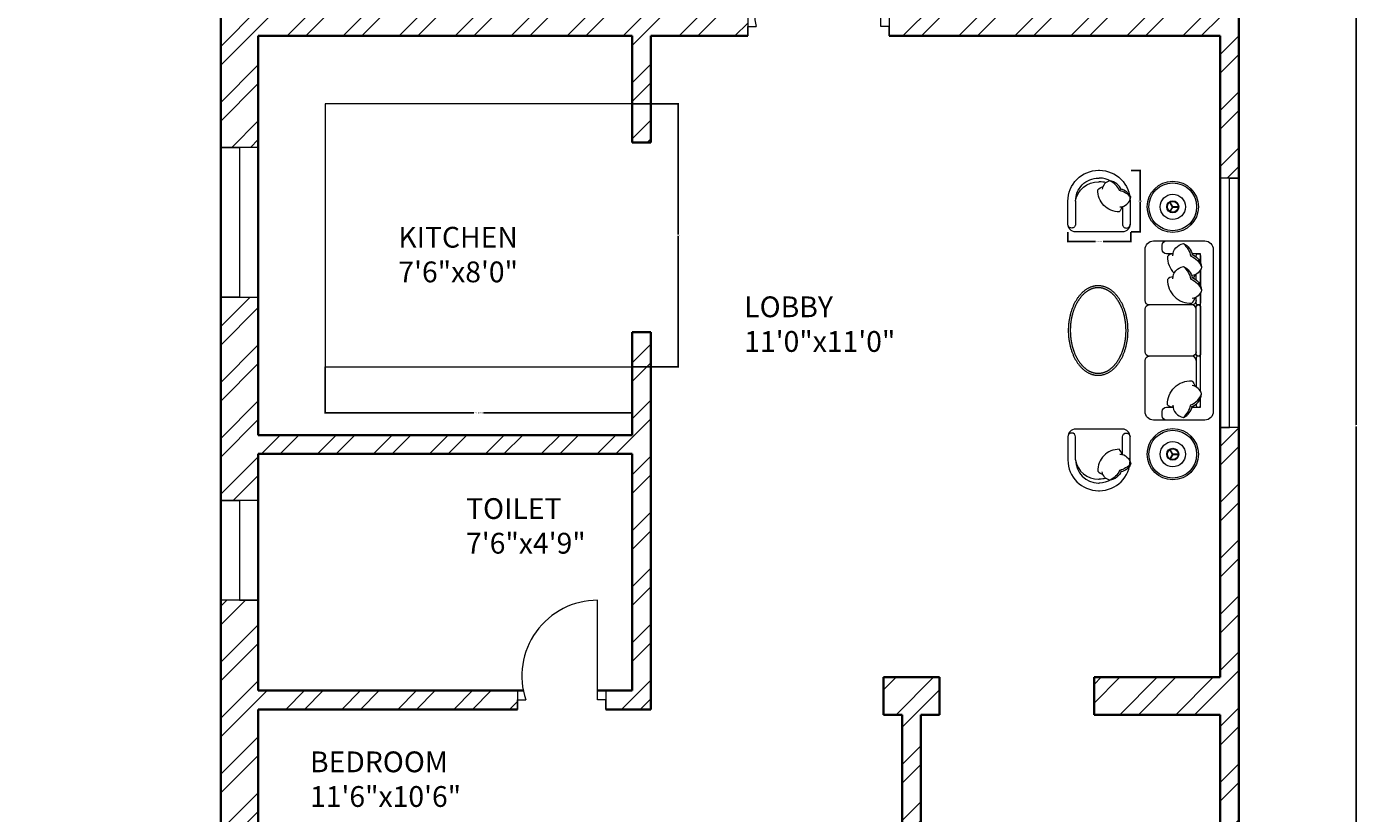
# Model space of a CAD drawing. Units: inches. Extents: x 1850 to 3445, y 1558 to 2756.
# Tile 6 of 13: x 2304 to 2625, y 1884 to 2073. Entities that reach past the tile are written whole.
import ezdxf

# ---------------------------------------------------------------- set-up
doc = ezdxf.new("R2010")
doc.units = ezdxf.units.IN
for name, color, linetype, lineweight in [('A-ANNO-DIMS', 2, 'Continuous', 18), ('A-AREA-IDEN', 7, 'Continuous', 18), ('A-DOOR', 3, 'Continuous', 18), ('A-FLOR-CASE', 8, 'Continuous', 18), ('A-FURN', 8, 'Continuous', 13), ('A-GLAZ', 4, 'Continuous', 18), ('A-WALL', 7, 'Continuous', 35), ('A-WALL-PATT', 252, 'Continuous', 13)]:
    doc.layers.add(name, color=color, linetype=linetype, lineweight=lineweight)
doc.styles.get("Standard").update_dxf_attribs({"font": 'arial.ttf'})
doc.dimstyles.get("Standard").update_dxf_attribs({"dimtxt": 0.18, "dimasz": 0.18, "dimexe": 0.18, "dimexo": 0.0625, "dimgap": 0.09, "dimtad": 0, "dimtih": 1, "dimtoh": 1, "dimdec": 4, "dimzin": 0, "dimdsep": 46, "dimtxsty": 'Standard', "dimcen": 0.09, "dimadec": 0, "dimazin": 0, "dimtfac": 1, "dimtdec": 4, "dimtofl": 0, "dimtmove": 0, "dimatfit": 3, "dimfxl": 1, "dimtolj": 1, "dimtzin": 0, "dimarcsym": 0})

# ---------------------------------------------------------------- blocks, each defined once
blk = doc.blocks.new('LAMP-ROUND-PLAN')
at = {"ltscale": 0.03}
for p, q in [((6.1, 6.13), (5.38, 7.38)), ((6.21, 6.19), (5.49, 7.44)), ((6.1, 6.19), (5.38, 4.94)), ((6.21, 6.13), (5.49, 4.87)), ((6.16, 6.22), (7.61, 6.22)), ((6.16, 6.09), (7.61, 6.09))]:
    blk.add_line(p, q, dxfattribs=at)
for radius in [6.16, 3.03, 1.45, 1.3]:
    blk.add_circle((6.16, 6.16), radius, dxfattribs=at)
blk.add_circle((6.16, 6.16), 5.75)
blk = doc.blocks.new('TABLE-COFFEE-OVAL')
at = {"ltscale": 0.03}
blk.add_polyline3d([(7.18, 0, 0), (7.32, 0, 0), (7.46, 0.01, 0), (7.59, 0.02, 0), (7.73, 0.03, 0), (7.86, 0.05, 0), (8, 0.07, 0), (8.13, 0.09, 0), (8.27, 0.12, 0), (8.4, 0.16, 0), (8.54, 0.19, 0), (8.67, 0.23, 0), (8.8, 0.28, 0), (8.93, 0.32, 0), (9.07, 0.38, 0), (9.2, 0.43, 0), (9.33, 0.49, 0), (9.46, 0.55, 0), (9.58, 0.62, 0), (9.71, 0.69, 0), (9.84, 0.76, 0), (9.96, 0.84, 0), (10.09, 0.92, 0), (10.21, 1.01, 0), (10.34, 1.09, 0), (10.46, 1.18, 0), (10.58, 1.28, 0), (10.7, 1.38, 0), (10.82, 1.48, 0), (10.93, 1.58, 0), (11.05, 1.69, 0), (11.16, 1.8, 0), (11.27, 1.92, 0), (11.38, 2.03, 0), (11.49, 2.16, 0), (11.6, 2.28, 0), (11.71, 2.41, 0), (11.81, 2.54, 0), (11.92, 2.67, 0), (12.02, 2.8, 0), (12.12, 2.94, 0), (12.22, 3.08, 0), (12.31, 3.23, 0), (12.41, 3.38, 0), (12.5, 3.53, 0), (12.59, 3.68, 0), (12.68, 3.83, 0), (12.76, 3.99, 0), (12.85, 4.15, 0), (12.93, 4.31, 0), (13.01, 4.48, 0), (13.09, 4.64, 0), (13.17, 4.81, 0), (13.24, 4.98, 0), (13.31, 5.15, 0), (13.38, 5.33, 0), (13.45, 5.51, 0), (13.52, 5.69, 0), (13.58, 5.87, 0), (13.64, 6.05, 0), (13.7, 6.23, 0), (13.75, 6.42, 0), (13.81, 6.61, 0), (13.86, 6.79, 0), (13.91, 6.98, 0), (13.96, 7.18, 0), (14, 7.37, 0), (14.04, 7.56, 0), (14.08, 7.76, 0), (14.12, 7.95, 0), (14.15, 8.15, 0), (14.18, 8.35, 0), (14.21, 8.55, 0), (14.24, 8.75, 0), (14.26, 8.95, 0), (14.29, 9.15, 0), (14.31, 9.35, 0), (14.32, 9.56, 0), (14.34, 9.76, 0), (14.35, 9.96, 0), (14.36, 10.17, 0), (14.36, 10.37, 0), (14.37, 10.57, 0), (14.37, 10.78, 0), (14.37, 10.98, 0), (14.36, 11.18, 0), (14.36, 11.39, 0), (14.35, 11.59, 0), (14.34, 11.8, 0), (14.32, 12, 0), (14.31, 12.2, 0), (14.29, 12.4, 0), (14.26, 12.6, 0), (14.24, 12.8, 0), (14.21, 13, 0), (14.18, 13.2, 0), (14.15, 13.4, 0), (14.12, 13.6, 0), (14.08, 13.8, 0), (14.04, 13.99, 0), (14, 14.18, 0), (13.96, 14.38, 0), (13.91, 14.57, 0), (13.86, 14.76, 0), (13.81, 14.95, 0), (13.75, 15.14, 0), (13.7, 15.32, 0), (13.64, 15.5, 0), (13.58, 15.69, 0), (13.52, 15.87, 0), (13.45, 16.05, 0), (13.38, 16.22, 0), (13.31, 16.4, 0), (13.24, 16.57, 0), (13.17, 16.74, 0), (13.09, 16.91, 0), (13.01, 17.08, 0), (12.93, 17.24, 0), (12.85, 17.4, 0), (12.76, 17.56, 0), (12.68, 17.72, 0), (12.59, 17.88, 0), (12.5, 18.03, 0), (12.41, 18.18, 0), (12.31, 18.32, 0), (12.22, 18.47, 0), (12.12, 18.61, 0), (12.02, 18.75, 0), (11.92, 18.88, 0), (11.81, 19.02, 0), (11.71, 19.15, 0), (11.6, 19.27, 0), (11.49, 19.4, 0), (11.38, 19.52, 0), (11.27, 19.64, 0), (11.16, 19.75, 0), (11.05, 19.86, 0), (10.93, 19.97, 0), (10.82, 20.08, 0), (10.7, 20.18, 0), (10.58, 20.27, 0), (10.46, 20.37, 0), (10.34, 20.46, 0), (10.21, 20.55, 0), (10.09, 20.63, 0), (9.96, 20.71, 0), (9.84, 20.79, 0), (9.71, 20.86, 0), (9.58, 20.93, 0), (9.46, 21, 0), (9.33, 21.06, 0), (9.2, 21.12, 0), (9.07, 21.18, 0), (8.93, 21.23, 0), (8.8, 21.28, 0), (8.67, 21.32, 0), (8.54, 21.36, 0), (8.4, 21.4, 0), (8.27, 21.43, 0), (8.13, 21.46, 0), (8, 21.48, 0), (7.86, 21.5, 0), (7.73, 21.52, 0), (7.59, 21.54, 0), (7.46, 21.55, 0), (7.32, 21.55, 0), (7.18, 21.55, 0), (7.05, 21.55, 0), (6.91, 21.55, 0), (6.78, 21.54, 0), (6.64, 21.52, 0), (6.5, 21.5, 0), (6.37, 21.48, 0), (6.23, 21.46, 0), (6.1, 21.43, 0), (5.97, 21.4, 0), (5.83, 21.36, 0), (5.7, 21.32, 0), (5.57, 21.28, 0), (5.43, 21.23, 0), (5.3, 21.18, 0), (5.17, 21.12, 0), (5.04, 21.06, 0), (4.91, 21, 0), (4.78, 20.93, 0), (4.66, 20.86, 0), (4.53, 20.79, 0), (4.4, 20.71, 0), (4.28, 20.63, 0), (4.15, 20.55, 0), (4.03, 20.46, 0), (3.91, 20.37, 0), (3.79, 20.27, 0), (3.67, 20.18, 0), (3.55, 20.08, 0), (3.44, 19.97, 0), (3.32, 19.86, 0), (3.21, 19.75, 0), (3.09, 19.64, 0), (2.98, 19.52, 0), (2.87, 19.4, 0), (2.77, 19.27, 0), (2.66, 19.15, 0), (2.55, 19.02, 0), (2.45, 18.88, 0), (2.35, 18.75, 0), (2.25, 18.61, 0), (2.15, 18.47, 0), (2.06, 18.32, 0), (1.96, 18.18, 0), (1.87, 18.03, 0), (1.78, 17.88, 0), (1.69, 17.72, 0), (1.6, 17.56, 0), (1.52, 17.4, 0), (1.44, 17.24, 0), (1.36, 17.08, 0), (1.28, 16.91, 0), (1.2, 16.74, 0), (1.13, 16.57, 0), (1.05, 16.4, 0), (0.98, 16.22, 0), (0.92, 16.05, 0), (0.85, 15.87, 0), (0.79, 15.69, 0), (0.73, 15.5, 0), (0.67, 15.32, 0), (0.61, 15.14, 0), (0.56, 14.95, 0), (0.51, 14.76, 0), (0.46, 14.57, 0), (0.41, 14.38, 0), (0.37, 14.18, 0), (0.33, 13.99, 0), (0.29, 13.8, 0), (0.25, 13.6, 0), (0.22, 13.4, 0), (0.18, 13.2, 0), (0.15, 13, 0), (0.13, 12.8, 0), (0.1, 12.6, 0), (0.08, 12.4, 0), (0.06, 12.2, 0), (0.05, 12, 0), (0.03, 11.8, 0), (0.02, 11.59, 0), (0.01, 11.39, 0), (0, 11.18, 0), (0, 10.98, 0), (0, 10.78, 0), (0, 10.57, 0), (0, 10.37, 0), (0.01, 10.17, 0), (0.02, 9.96, 0), (0.03, 9.76, 0), (0.05, 9.56, 0), (0.06, 9.35, 0), (0.08, 9.15, 0), (0.1, 8.95, 0), (0.13, 8.75, 0), (0.15, 8.55, 0), (0.18, 8.35, 0), (0.22, 8.15, 0), (0.25, 7.95, 0), (0.29, 7.76, 0), (0.33, 7.56, 0), (0.37, 7.37, 0), (0.41, 7.18, 0), (0.46, 6.98, 0), (0.51, 6.79, 0), (0.56, 6.61, 0), (0.61, 6.42, 0), (0.67, 6.23, 0), (0.73, 6.05, 0), (0.79, 5.87, 0), (0.85, 5.69, 0), (0.92, 5.51, 0), (0.98, 5.33, 0), (1.05, 5.15, 0), (1.13, 4.98, 0), (1.2, 4.81, 0), (1.28, 4.64, 0), (1.36, 4.48, 0), (1.44, 4.31, 0), (1.52, 4.15, 0), (1.6, 3.99, 0), (1.69, 3.83, 0), (1.78, 3.68, 0), (1.87, 3.53, 0), (1.96, 3.38, 0), (2.06, 3.23, 0), (2.15, 3.08, 0), (2.25, 2.94, 0), (2.35, 2.8, 0), (2.45, 2.67, 0), (2.55, 2.54, 0), (2.66, 2.41, 0), (2.77, 2.28, 0), (2.87, 2.16, 0), (2.98, 2.03, 0), (3.09, 1.92, 0), (3.21, 1.8, 0), (3.32, 1.69, 0), (3.44, 1.58, 0), (3.55, 1.48, 0), (3.67, 1.38, 0), (3.79, 1.28, 0), (3.91, 1.18, 0), (4.03, 1.09, 0), (4.15, 1.01, 0), (4.28, 0.92, 0), (4.4, 0.84, 0), (4.53, 0.76, 0), (4.66, 0.69, 0), (4.78, 0.62, 0), (4.91, 0.55, 0), (5.04, 0.49, 0), (5.17, 0.43, 0), (5.3, 0.38, 0), (5.43, 0.32, 0), (5.57, 0.28, 0), (5.7, 0.23, 0), (5.83, 0.19, 0), (5.97, 0.16, 0), (6.1, 0.12, 0), (6.23, 0.09, 0), (6.37, 0.07, 0), (6.5, 0.05, 0), (6.64, 0.03, 0), (6.78, 0.02, 0), (6.91, 0.01, 0), (7.05, 0, 0), (7.18, 0, 0)], dxfattribs=at)
blk.add_polyline3d([(7.18, 0.48, 0), (7.26, 0.48, 0), (7.33, 0.48, 0), (7.41, 0.49, 0), (7.48, 0.49, 0), (7.55, 0.5, 0), (7.63, 0.5, 0), (7.7, 0.51, 0), (7.78, 0.52, 0), (7.86, 0.53, 0), (7.93, 0.54, 0), (8.01, 0.56, 0), (8.09, 0.57, 0), (8.16, 0.59, 0), (8.24, 0.61, 0), (8.32, 0.63, 0), (8.39, 0.65, 0), (8.47, 0.67, 0), (8.55, 0.7, 0), (8.63, 0.72, 0), (8.71, 0.75, 0), (8.78, 0.78, 0), (8.86, 0.81, 0), (8.94, 0.84, 0), (9.02, 0.88, 0), (9.1, 0.91, 0), (9.18, 0.95, 0), (9.26, 0.99, 0), (9.33, 1.03, 0), (9.41, 1.07, 0), (9.49, 1.12, 0), (9.57, 1.16, 0), (9.65, 1.21, 0), (9.73, 1.26, 0), (9.8, 1.31, 0), (9.88, 1.36, 0), (9.96, 1.41, 0), (10.04, 1.47, 0), (10.11, 1.53, 0), (10.19, 1.58, 0), (10.27, 1.64, 0), (10.34, 1.71, 0), (10.42, 1.77, 0), (10.5, 1.84, 0), (10.57, 1.9, 0), (10.65, 1.97, 0), (10.72, 2.04, 0), (10.79, 2.12, 0), (10.87, 2.19, 0), (10.94, 2.27, 0), (11.01, 2.34, 0), (11.09, 2.42, 0), (11.16, 2.5, 0), (11.23, 2.58, 0), (11.3, 2.67, 0), (11.37, 2.75, 0), (11.44, 2.84, 0), (11.5, 2.93, 0), (11.57, 3.02, 0), (11.64, 3.11, 0), (11.71, 3.2, 0), (11.77, 3.3, 0), (11.84, 3.39, 0), (11.9, 3.49, 0), (11.96, 3.59, 0), (12.03, 3.68, 0), (12.09, 3.78, 0), (12.15, 3.89, 0), (12.21, 3.99, 0), (12.27, 4.09, 0), (12.33, 4.2, 0), (12.38, 4.3, 0), (12.44, 4.41, 0), (12.5, 4.52, 0), (12.55, 4.63, 0), (12.6, 4.74, 0), (12.66, 4.85, 0), (12.71, 4.96, 0), (12.76, 5.08, 0), (12.81, 5.19, 0), (12.86, 5.3, 0), (12.9, 5.42, 0), (12.95, 5.54, 0), (12.99, 5.65, 0), (13.04, 5.77, 0), (13.08, 5.89, 0), (13.12, 6.01, 0), (13.16, 6.13, 0), (13.2, 6.25, 0), (13.24, 6.37, 0), (13.28, 6.49, 0), (13.31, 6.61, 0), (13.35, 6.73, 0), (13.38, 6.85, 0), (13.41, 6.97, 0), (13.44, 7.09, 0), (13.47, 7.21, 0), (13.5, 7.34, 0), (13.53, 7.46, 0), (13.56, 7.58, 0), (13.58, 7.7, 0), (13.61, 7.83, 0), (13.63, 7.95, 0), (13.65, 8.07, 0), (13.68, 8.19, 0), (13.7, 8.32, 0), (13.72, 8.44, 0), (13.73, 8.56, 0), (13.75, 8.69, 0), (13.77, 8.81, 0), (13.78, 8.94, 0), (13.8, 9.06, 0), (13.81, 9.19, 0), (13.82, 9.31, 0), (13.83, 9.43, 0), (13.84, 9.56, 0), (13.85, 9.68, 0), (13.86, 9.81, 0), (13.87, 9.93, 0), (13.87, 10.06, 0), (13.88, 10.18, 0), (13.88, 10.31, 0), (13.89, 10.43, 0), (13.89, 10.56, 0), (13.89, 10.68, 0), (13.89, 10.81, 0), (13.89, 10.93, 0), (13.89, 11.06, 0), (13.88, 11.18, 0), (13.88, 11.31, 0), (13.88, 11.43, 0), (13.87, 11.56, 0), (13.86, 11.68, 0), (13.86, 11.81, 0), (13.85, 11.93, 0), (13.84, 12.06, 0), (13.83, 12.18, 0), (13.82, 12.31, 0), (13.8, 12.43, 0), (13.79, 12.55, 0), (13.77, 12.68, 0), (13.76, 12.8, 0), (13.74, 12.93, 0), (13.72, 13.05, 0), (13.71, 13.17, 0), (13.69, 13.3, 0), (13.66, 13.42, 0), (13.64, 13.54, 0), (13.62, 13.67, 0), (13.6, 13.79, 0), (13.57, 13.91, 0), (13.54, 14.03, 0), (13.52, 14.16, 0), (13.49, 14.28, 0), (13.46, 14.4, 0), (13.43, 14.52, 0), (13.4, 14.64, 0), (13.36, 14.76, 0), (13.33, 14.88, 0), (13.29, 15.01, 0), (13.26, 15.13, 0), (13.22, 15.25, 0), (13.18, 15.36, 0), (13.14, 15.48, 0), (13.1, 15.6, 0), (13.06, 15.72, 0), (13.02, 15.84, 0), (12.97, 15.96, 0), (12.93, 16.07, 0), (12.88, 16.19, 0), (12.83, 16.31, 0), (12.78, 16.42, 0), (12.73, 16.53, 0), (12.68, 16.65, 0), (12.63, 16.76, 0), (12.58, 16.87, 0), (12.52, 16.98, 0), (12.47, 17.09, 0), (12.41, 17.2, 0), (12.36, 17.3, 0), (12.3, 17.41, 0), (12.24, 17.51, 0), (12.18, 17.62, 0), (12.12, 17.72, 0), (12.06, 17.82, 0), (12, 17.92, 0), (11.93, 18.02, 0), (11.87, 18.11, 0), (11.8, 18.21, 0), (11.74, 18.3, 0), (11.67, 18.4, 0), (11.61, 18.49, 0), (11.54, 18.58, 0), (11.47, 18.67, 0), (11.4, 18.76, 0), (11.33, 18.84, 0), (11.26, 18.93, 0), (11.19, 19.01, 0), (11.12, 19.09, 0), (11.05, 19.17, 0), (10.98, 19.25, 0), (10.9, 19.33, 0), (10.83, 19.4, 0), (10.76, 19.47, 0), (10.68, 19.55, 0), (10.61, 19.62, 0), (10.53, 19.68, 0), (10.46, 19.75, 0), (10.38, 19.82, 0), (10.31, 19.88, 0), (10.23, 19.94, 0), (10.15, 20, 0), (10.08, 20.06, 0), (10, 20.11, 0), (9.92, 20.17, 0), (9.84, 20.22, 0), (9.77, 20.27, 0), (9.69, 20.32, 0), (9.61, 20.37, 0), (9.53, 20.42, 0), (9.45, 20.46, 0), (9.37, 20.5, 0), (9.3, 20.54, 0), (9.22, 20.58, 0), (9.14, 20.62, 0), (9.06, 20.66, 0), (8.98, 20.69, 0), (8.9, 20.73, 0), (8.82, 20.76, 0), (8.75, 20.79, 0), (8.67, 20.82, 0), (8.59, 20.84, 0), (8.51, 20.87, 0), (8.43, 20.89, 0), (8.36, 20.91, 0), (8.28, 20.93, 0), (8.2, 20.95, 0), (8.12, 20.97, 0), (8.05, 20.99, 0), (7.97, 21, 0), (7.89, 21.02, 0), (7.82, 21.03, 0), (7.74, 21.04, 0), (7.67, 21.05, 0), (7.59, 21.05, 0), (7.52, 21.06, 0), (7.44, 21.07, 0), (7.37, 21.07, 0), (7.29, 21.07, 0), (7.22, 21.07, 0), (7.15, 21.07, 0), (7.07, 21.07, 0), (7, 21.07, 0), (6.93, 21.07, 0), (6.85, 21.06, 0), (6.78, 21.05, 0), (6.7, 21.05, 0), (6.62, 21.04, 0), (6.55, 21.03, 0), (6.47, 21.02, 0), (6.4, 21, 0), (6.32, 20.99, 0), (6.24, 20.97, 0), (6.17, 20.95, 0), (6.09, 20.93, 0), (6.01, 20.91, 0), (5.93, 20.89, 0), (5.86, 20.87, 0), (5.78, 20.84, 0), (5.7, 20.82, 0), (5.62, 20.79, 0), (5.54, 20.76, 0), (5.47, 20.73, 0), (5.39, 20.69, 0), (5.31, 20.66, 0), (5.23, 20.62, 0), (5.15, 20.58, 0), (5.07, 20.54, 0), (4.99, 20.5, 0), (4.92, 20.46, 0), (4.84, 20.42, 0), (4.76, 20.37, 0), (4.68, 20.32, 0), (4.6, 20.27, 0), (4.52, 20.22, 0), (4.45, 20.17, 0), (4.37, 20.11, 0), (4.29, 20.06, 0), (4.21, 20, 0), (4.14, 19.94, 0), (4.06, 19.88, 0), (3.98, 19.82, 0), (3.91, 19.75, 0), (3.83, 19.68, 0), (3.76, 19.62, 0), (3.68, 19.55, 0), (3.61, 19.47, 0), (3.54, 19.4, 0), (3.46, 19.33, 0), (3.39, 19.25, 0), (3.32, 19.17, 0), (3.25, 19.09, 0), (3.18, 19.01, 0), (3.11, 18.93, 0), (3.04, 18.84, 0), (2.97, 18.76, 0), (2.9, 18.67, 0), (2.83, 18.58, 0), (2.76, 18.49, 0), (2.69, 18.4, 0), (2.63, 18.3, 0), (2.56, 18.21, 0), (2.5, 18.11, 0), (2.44, 18.02, 0), (2.37, 17.92, 0), (2.31, 17.82, 0), (2.25, 17.72, 0), (2.19, 17.62, 0), (2.13, 17.51, 0), (2.07, 17.41, 0), (2.01, 17.3, 0), (1.96, 17.2, 0), (1.9, 17.09, 0), (1.84, 16.98, 0), (1.79, 16.87, 0), (1.74, 16.76, 0), (1.69, 16.65, 0), (1.63, 16.53, 0), (1.58, 16.42, 0), (1.54, 16.31, 0), (1.49, 16.19, 0), (1.44, 16.07, 0), (1.4, 15.96, 0), (1.35, 15.84, 0), (1.31, 15.72, 0), (1.27, 15.6, 0), (1.23, 15.48, 0), (1.19, 15.36, 0), (1.15, 15.25, 0), (1.11, 15.13, 0), (1.07, 15.01, 0), (1.04, 14.88, 0), (1, 14.76, 0), (0.97, 14.64, 0), (0.94, 14.52, 0), (0.91, 14.4, 0), (0.88, 14.28, 0), (0.85, 14.16, 0), (0.82, 14.03, 0), (0.8, 13.91, 0), (0.77, 13.79, 0), (0.75, 13.67, 0), (0.72, 13.54, 0), (0.7, 13.42, 0), (0.68, 13.3, 0), (0.66, 13.17, 0), (0.64, 13.05, 0), (0.63, 12.93, 0), (0.61, 12.8, 0), (0.59, 12.68, 0), (0.58, 12.55, 0), (0.56, 12.43, 0), (0.55, 12.31, 0), (0.54, 12.18, 0), (0.53, 12.06, 0), (0.52, 11.93, 0), (0.51, 11.81, 0), (0.5, 11.68, 0), (0.5, 11.56, 0), (0.49, 11.43, 0), (0.49, 11.31, 0), (0.48, 11.18, 0), (0.48, 11.06, 0), (0.48, 10.93, 0), (0.48, 10.81, 0), (0.48, 10.68, 0), (0.48, 10.56, 0), (0.48, 10.43, 0), (0.49, 10.31, 0), (0.49, 10.18, 0), (0.49, 10.06, 0), (0.5, 9.93, 0), (0.51, 9.81, 0), (0.52, 9.68, 0), (0.52, 9.56, 0), (0.53, 9.43, 0), (0.55, 9.31, 0), (0.56, 9.19, 0), (0.57, 9.06, 0), (0.59, 8.94, 0), (0.6, 8.81, 0), (0.62, 8.69, 0), (0.63, 8.56, 0), (0.65, 8.44, 0), (0.67, 8.32, 0), (0.69, 8.19, 0), (0.71, 8.07, 0), (0.74, 7.95, 0), (0.76, 7.83, 0), (0.78, 7.7, 0), (0.81, 7.58, 0), (0.84, 7.46, 0), (0.86, 7.34, 0), (0.89, 7.21, 0), (0.92, 7.09, 0), (0.96, 6.97, 0), (0.99, 6.85, 0), (1.02, 6.73, 0), (1.06, 6.61, 0), (1.09, 6.49, 0), (1.13, 6.37, 0), (1.17, 6.25, 0), (1.21, 6.13, 0), (1.25, 6.01, 0), (1.29, 5.89, 0), (1.33, 5.77, 0), (1.37, 5.65, 0), (1.42, 5.54, 0), (1.46, 5.42, 0), (1.51, 5.3, 0), (1.56, 5.19, 0), (1.61, 5.08, 0), (1.66, 4.96, 0), (1.71, 4.85, 0), (1.76, 4.74, 0), (1.82, 4.63, 0), (1.87, 4.52, 0), (1.93, 4.41, 0), (1.98, 4.3, 0), (2.04, 4.2, 0), (2.1, 4.09, 0), (2.16, 3.99, 0), (2.22, 3.89, 0), (2.28, 3.78, 0), (2.34, 3.68, 0), (2.4, 3.59, 0), (2.47, 3.49, 0), (2.53, 3.39, 0), (2.6, 3.3, 0), (2.66, 3.2, 0), (2.73, 3.11, 0), (2.8, 3.02, 0), (2.86, 2.93, 0), (2.93, 2.84, 0), (3, 2.75, 0), (3.07, 2.67, 0), (3.14, 2.58, 0), (3.21, 2.5, 0), (3.28, 2.42, 0), (3.35, 2.34, 0), (3.43, 2.27, 0), (3.5, 2.19, 0), (3.57, 2.12, 0), (3.65, 2.04, 0), (3.72, 1.97, 0), (3.8, 1.9, 0), (3.87, 1.84, 0), (3.95, 1.77, 0), (4.02, 1.71, 0), (4.1, 1.64, 0), (4.18, 1.58, 0), (4.25, 1.53, 0), (4.33, 1.47, 0), (4.41, 1.41, 0), (4.48, 1.36, 0), (4.56, 1.31, 0), (4.64, 1.26, 0), (4.72, 1.21, 0), (4.8, 1.16, 0), (4.88, 1.12, 0), (4.95, 1.07, 0), (5.03, 1.03, 0), (5.11, 0.99, 0), (5.19, 0.95, 0), (5.27, 0.91, 0), (5.35, 0.88, 0), (5.43, 0.84, 0), (5.5, 0.81, 0), (5.58, 0.78, 0), (5.66, 0.75, 0), (5.74, 0.72, 0), (5.82, 0.7, 0), (5.9, 0.67, 0), (5.97, 0.65, 0), (6.05, 0.63, 0), (6.13, 0.61, 0), (6.21, 0.59, 0), (6.28, 0.57, 0), (6.36, 0.56, 0), (6.43, 0.54, 0), (6.51, 0.53, 0), (6.59, 0.52, 0), (6.66, 0.51, 0), (6.74, 0.5, 0), (6.81, 0.5, 0), (6.89, 0.49, 0), (6.96, 0.49, 0), (7.04, 0.48, 0), (7.11, 0.48, 0), (7.18, 0.48, 0)])
blk = doc.blocks.new('CHAIR-LOUNGE-CUSHION')
at = {"ltscale": 0.03}
blk.add_lwpolyline([(7.5, 0), (1.85, 0, -0.414214), (0, 1.85), (0, 7.4, -0.414214), (7.4, 14.81), (7.5, 14.81), (7.59, 14.81, -0.414214), (14.99, 7.4), (14.99, 1.85, -0.414214), (13.14, 0), (7.5, 0)], format="xyb", dxfattribs=at)
for points in [[(1.85, 7.4, -0.414214), (7.4, 12.95), (7.5, 12.95)], [(10.34, 12.22, 0.130591), (7.59, 12.95), (7.5, 12.95)], [(1.85, 7.4, -0.372719), (7.4, 12.03), (7.5, 12.03)], [(12.96, 6.06, -0.165541), (12.38, 4.84, -0.425989), (7.19, 10.14, -0.121523), (8.42, 10.87, 7.115464)], [(9.17, 11.83, 0.072384), (7.59, 12.03), (7.5, 12.03)], [(12.81, 10.05, 0.306663), (10.05, 12.26, 0.30633), (8.25, 10.25, -0.872847)], [(15.14, 8.34, 0.14773), (12.44, 9.93, 0.213343), (10.05, 12.26, 0.178662)], [(12.49, 6, 0.356772), (15.14, 8.34, 0.249542), (12.74, 10.26, -9.61688)], [(1.85, 7.4), (1.85, 1.85, -0.414214), (0.92, 0.93), (0.92, 0.93, -0.414214), (0, 1.85)], [(13.14, 6.11), (13.14, 1.85, 0.414214), (14.07, 0.93), (14.07, 0.93, 0.414214), (14.99, 1.85)]]:
    blk.add_lwpolyline(points, format="xyb")
blk = doc.blocks.new('WIN-36-W9-ALT')
for p, q in [((9, 36), (0, 36)), ((0, 36), (4.5, 36)), ((4.5, 36), (4.5, 0)), ((4.5, 0), (0, 0)), ((0, 0), (9, 0))]:
    blk.add_line(p, q)
blk = doc.blocks.new('WIN-24-W9')
for p, q in [((9, 24), (0, 24)), ((0, 24), (4.5, 24)), ((4.5, 24), (4.5, 0)), ((9, 0), (0, 0)), ((4.5, 0), (9, 0))]:
    blk.add_line(p, q)
blk = doc.blocks.new('WIN-60-W4_5')
for p, q in [((0, 60), (4.5, 60)), ((4.5, 60), (2.25, 60)), ((2.25, 60), (2.25, 0)), ((2.25, 0), (0, 0)), ((0, 0), (4.5, 0))]:
    blk.add_line(p, q)
blk = doc.blocks.new('DOOR-BED-UPPER')
for p, q in [((32.07, 2.25), (32.07, 38.25)), ((0, 4.5), (0, 0)), ((34.07, 4.5), (34.07, 0)), ((0, 0), (0, 2.25)), ((0, 2.25), (2, 2.25)), ((34.07, 2.25), (32.07, 2.25)), ((34.07, 0), (34.07, 2.25))]:
    blk.add_line(p, q)
blk.add_arc((32.07, 7.69), 30.56, 90, 190.2532)
blk = doc.blocks.new('DOOR-BATH-LOWER-HALL')
for p, q in [((19.31, 2.25), (19.31, 26.25)), ((0, 4.5), (0, 0)), ((21.31, 4.5), (21.31, 0)), ((0, 0), (0, 2.25)), ((0, 2.25), (2, 2.25)), ((21.31, 2.25), (19.31, 2.25)), ((21.31, 0), (21.31, 2.25))]:
    blk.add_line(p, q)
blk.add_arc((19.31, 8.01), 18.24, 90, 198.4026)
blk = doc.blocks.new('COUNTER-U-UPPER')
for p, q in [((73.88, 63.24), (0, 63.24)), ((0, 63.24), (0, 0)), ((0, 0), (73.88, 0))]:
    blk.add_line(p, q)
blk = doc.blocks.new('*D54')
at = {"layer": 'A-ANNO-DIMS', "color": 0, "lineweight": -2, "transparency": 16777216}
for p, q in [((2554.92, 2023.49), (2554.92, 2021.1)), ((2555.1, 2021.28), (2561.54, 2021.28)), ((2569.89, 2021.28), (2563.45, 2021.28)), ((2570.07, 2023.49), (2570.07, 2021.1))]:
    blk.add_line(p, q, dxfattribs=at)
at = {"layer": 'A-ANNO-DIMS', "color": 0, "transparency": 16777216}
for points in [[(2555.1, 2021.31), (2555.1, 2021.25), (2554.92, 2021.28)], [(2569.89, 2021.31), (2569.89, 2021.25), (2570.07, 2021.28)]]:
    blk.add_solid(points, dxfattribs=at)
at = {"layer": 'Defpoints', "color": 0, "transparency": 16777216}
for p in [(2554.92, 2023.55), (2570.07, 2023.55), (2570.07, 2021.28)]:
    blk.add_point(p, dxfattribs=at)
at = {"layer": 'A-ANNO-DIMS', "color": 0, "transparency": 16777216, "insert": (2562.49, 2021.28), "char_height": 0.18, "attachment_point": 5}
blk.add_mtext('\\A1;CHAIR 15 TYP.', dxfattribs=at)
blk = doc.blocks.new('*D55')
at = {"layer": 'A-ANNO-DIMS', "color": 0, "lineweight": -2, "transparency": 16777216}
for p, q in [((2570.13, 2038.36), (2572.52, 2038.36)), ((2572.34, 2038.18), (2572.34, 2031.14)), ((2572.34, 2023.73), (2572.34, 2030.77)), ((2570.13, 2023.55), (2572.52, 2023.55))]:
    blk.add_line(p, q, dxfattribs=at)
at = {"layer": 'A-ANNO-DIMS', "color": 0, "transparency": 16777216}
for points in [[(2572.31, 2038.18), (2572.37, 2038.18), (2572.34, 2038.36)], [(2572.31, 2023.73), (2572.37, 2023.73), (2572.34, 2023.55)]]:
    blk.add_solid(points, dxfattribs=at)
at = {"layer": 'Defpoints', "color": 0, "transparency": 16777216}
for p in [(2570.07, 2038.36), (2572.34, 2038.36), (2570.07, 2023.55)]:
    blk.add_point(p, dxfattribs=at)
at = {"layer": 'A-ANNO-DIMS', "color": 0, "transparency": 16777216, "insert": (2572.34, 2030.95), "char_height": 0.18, "attachment_point": 5}
blk.add_mtext('\\A1;15 TYP.', dxfattribs=at)
blk = doc.blocks.new('*D74')
at = {"layer": 'A-ANNO-DIMS', "color": 0, "lineweight": -2, "transparency": 16777216}
for p, q in [((2376.18, 1991.05), (2376.18, 1979.85)), ((2450.06, 1991.05), (2450.06, 1979.85)), ((2376.36, 1980.03), (2411.93, 1980.03)), ((2449.88, 1980.03), (2414.3, 1980.03))]:
    blk.add_line(p, q, dxfattribs=at)
at = {"layer": 'A-ANNO-DIMS', "color": 0, "transparency": 16777216}
for points in [[(2376.36, 1980.06), (2376.36, 1980), (2376.18, 1980.03)], [(2449.88, 1980.06), (2449.88, 1980), (2450.06, 1980.03)]]:
    blk.add_solid(points, dxfattribs=at)
at = {"layer": 'Defpoints', "color": 0, "transparency": 16777216}
for p in [(2376.18, 1991.11), (2450.06, 1991.11), (2450.06, 1980.03)]:
    blk.add_point(p, dxfattribs=at)
at = {"layer": 'A-ANNO-DIMS', "color": 0, "transparency": 16777216, "insert": (2413.12, 1980.03), "char_height": 0.18, "attachment_point": 5}
blk.add_mtext('\\A1;COUNTER 74 TYP.', dxfattribs=at)
blk = doc.blocks.new('*D75')
at = {"layer": 'A-ANNO-DIMS', "color": 0, "lineweight": -2, "transparency": 16777216}
for p, q in [((2450.12, 2054.35), (2461.32, 2054.35)), ((2461.14, 2054.17), (2461.14, 2022.92)), ((2461.14, 1991.29), (2461.14, 2022.55)), ((2450.12, 1991.11), (2461.32, 1991.11))]:
    blk.add_line(p, q, dxfattribs=at)
at = {"layer": 'A-ANNO-DIMS', "color": 0, "transparency": 16777216}
for points in [[(2461.11, 2054.17), (2461.17, 2054.17), (2461.14, 2054.35)], [(2461.11, 1991.29), (2461.17, 1991.29), (2461.14, 1991.11)]]:
    blk.add_solid(points, dxfattribs=at)
at = {"layer": 'Defpoints', "color": 0, "transparency": 16777216}
for p in [(2450.06, 2054.35), (2461.14, 2054.35), (2450.06, 1991.11)]:
    blk.add_point(p, dxfattribs=at)
at = {"layer": 'A-ANNO-DIMS', "color": 0, "transparency": 16777216, "insert": (2461.14, 2022.73), "char_height": 0.18, "attachment_point": 5}
blk.add_mtext('\\A1;63 TYP.', dxfattribs=at)
blk = doc.blocks.new('*D83')
at = {"layer": 'A-ANNO-DIMS', "color": 0, "lineweight": -2, "transparency": 16777216}
for p, q in [((2596.12, 2216.18), (2624.49, 2216.18)), ((2624.31, 2216), (2624.31, 1977.12)), ((2624.31, 1737.86), (2624.31, 1976.75)), ((2596.12, 1737.68), (2624.49, 1737.68))]:
    blk.add_line(p, q, dxfattribs=at)
at = {"layer": 'A-ANNO-DIMS', "color": 0, "transparency": 16777216}
for points in [[(2624.28, 2216), (2624.34, 2216), (2624.31, 2216.18)], [(2624.28, 1737.86), (2624.34, 1737.86), (2624.31, 1737.68)]]:
    blk.add_solid(points, dxfattribs=at)
at = {"layer": 'Defpoints', "color": 0, "transparency": 16777216}
for p in [(2596.06, 2216.18), (2624.31, 2216.18), (2596.06, 1737.68)]:
    blk.add_point(p, dxfattribs=at)
at = {"layer": 'A-ANNO-DIMS', "color": 0, "transparency": 16777216, "insert": (2624.31, 1976.93), "char_height": 0.18, "attachment_point": 5}
blk.add_mtext('\\A1;478.5', dxfattribs=at)

msp = doc.modelspace()

# ---------------------------------------------------------------- hatches: boundary and pattern name
at = {"layer": 'A-WALL-PATT'}
h = msp.add_hatch(dxfattribs=at)
h.set_pattern_fill('ANSI32', color=256)
h.paths.add_polyline_path([(2519.5556, 1907.3936), (2523.9987, 1907.3936), (2523.9987, 1916.3936), (2519.5556, 1916.3936), (2515.0556, 1916.3936), (2510.5556, 1916.3936), (2510.5556, 1907.3936), (2515.0556, 1907.3936), (2515.0556, 1742.1843), (2515.0556, 1737.6843), (2596.0556, 1737.6843), (2596.0556, 1976.4962), (2591.5556, 1976.4962), (2591.5556, 1916.3936), (2561.2666, 1916.3936), (2561.2666, 1907.3936), (2591.5556, 1907.3936), (2591.5556, 1746.6843), (2519.5556, 1746.6843)])
h.paths.add_polyline_path([(2076.6481, 2211.6843), (2076.6481, 2216.1843), (2040.2715, 2216.1843), (2040.2715, 2175.83), (2044.7715, 2175.83), (2049.2715, 2175.83), (2049.2715, 2207.1843), (2076.6481, 2207.1843)])
h.paths.add_polyline_path([(2211.7715, 2216.1843), (2136.6481, 2216.1843), (2136.6481, 2207.1843), (2211.7715, 2207.1843)])
h.paths.add_polyline_path([(2285.2715, 2154.1843), (2250.6169, 2154.1843), (2250.6169, 2149.6843), (2280.7715, 2149.6843), (2280.7715, 2075.1843), (2236.3632, 2075.1843), (2236.3632, 2070.6843), (2285.2715, 2070.6843)])
h.paths.add_polyline_path([(2228.3485, 2154.1843), (2207.2715, 2154.1843), (2207.2715, 2075.1843), (2201.9819, 2075.1843), (2201.9819, 2070.6843), (2215.4663, 2070.6843), (2215.4663, 2072.9343), (2215.4663, 2075.1843), (2211.7715, 2075.1843), (2211.7715, 2149.6843), (2228.3485, 2149.6843)])
h.paths.add_polyline_path([(2049.2715, 2115.83), (2040.2715, 2115.83), (2040.2715, 2042.8465), (2049.2715, 2042.8465), (2049.2715, 2070.6843), (2168.6057, 2070.6843), (2168.6057, 2072.9343), (2168.6057, 2075.1843), (2049.2715, 2075.1843)])
h.paths.add_polyline_path([(2049.2715, 1982.8465), (2040.2715, 1982.8465), (2040.2715, 1910.2175), (2060.9481, 1910.2175), (2060.9481, 1914.7175), (2060.9481, 1919.2175), (2049.2715, 1919.2175)])
h.paths.add_polyline_path([(2132.4938, 1919.2175), (2108.9481, 1919.2175), (2108.9481, 1910.2175), (2132.4938, 1910.2175), (2132.4938, 1914.6749)])
h.paths.add_polyline_path([(2178.7715, 1938.6843), (2169.7715, 1938.6843), (2169.7715, 1919.2175), (2163.687, 1919.2175), (2163.687, 1910.2175), (2169.7715, 1910.2175), (2169.7715, 1854.6843), (2169.7715, 1845.6843), (2196.1287, 1845.6843), (2196.1287, 1850.1843), (2196.1287, 1854.6843), (2178.7715, 1854.6843)])
h.paths.add_polyline_path([(2049.2715, 1910.2175), (2040.2715, 1910.2175), (2040.2715, 1745.6843), (2049.2715, 1745.6843)])
h.paths.add_polyline_path([(2146.8861, 1766.7204), (2159.0894, 1766.7204), (2159.0894, 1777.0239), (2146.8861, 1777.0239)], flags=9)
h.paths.add_polyline_path([(2183.4664, 1798.4016), (2226.7338, 1798.4016), (2226.7338, 1817.0589), (2183.4664, 1817.0589)], flags=9)
h.paths.add_polyline_path([(2070.863, 1867.537), (2109.9796, 1867.537), (2109.9796, 1886.1943), (2070.863, 1886.1943)], flags=9)
h = msp.add_hatch(dxfattribs=at)
h.set_pattern_fill('ANSI32', color=256)
h.paths.add_polyline_path([(2403.5576, 2211.6843), (2403.5576, 2216.1843), (2351.0556, 2216.1843), (2351.0556, 2169.0079), (2360.0556, 2169.0079), (2360.0556, 2207.1843), (2403.5576, 2207.1843)])
h.paths.add_polyline_path([(2522.5556, 2216.1843), (2463.5576, 2216.1843), (2463.5576, 2207.1843), (2522.5556, 2207.1843)])
h.paths.add_polyline_path([(2596.0556, 2154.1843), (2562.6647, 2154.1843), (2562.6647, 2149.6843), (2591.5556, 2149.6843), (2591.5556, 2075.1843), (2522.5556, 2075.1843), (2522.5556, 2079.8699), (2518.0556, 2079.8699), (2518.0556, 2075.1843), (2511.9412, 2075.1843), (2511.9412, 2070.6843), (2591.5556, 2070.6843), (2591.5556, 2036.4962), (2596.0556, 2036.4962)])
h.paths.add_polyline_path([(2538.6647, 2154.1843), (2522.5556, 2154.1843), (2518.0556, 2154.1843), (2518.0556, 2102.7998), (2522.5556, 2102.7998), (2522.5556, 2149.6843), (2538.6647, 2149.6843)], flags=17)
h.paths.add_polyline_path([(2477.8689, 2072.9343), (2477.8689, 2075.1843), (2360.0556, 2075.1843), (2360.0556, 2109.0079), (2355.5556, 2109.0079), (2351.0556, 2109.0079), (2351.0556, 2043.8694), (2355.5556, 2043.8694), (2360.0556, 2043.8694), (2360.0556, 2070.6843), (2450.0556, 2070.6843), (2450.0556, 2045.0271), (2454.5556, 2045.0271), (2454.5556, 2070.6843), (2477.8689, 2070.6843)])
h.paths.add_polyline_path([(2360.0556, 2007.8694), (2351.0556, 2007.8694), (2351.0556, 1958.9131), (2355.5556, 1958.9131), (2360.0556, 1958.9131), (2360.0556, 1970.1843), (2450.0556, 1970.1843), (2450.0556, 1913.1843), (2443.7332, 1913.1843), (2443.7332, 1908.6843), (2454.5556, 1908.6843), (2454.5556, 1999.4184), (2450.0556, 1999.4184), (2450.0556, 1974.6843), (2360.0556, 1974.6843)])
h.paths.add_polyline_path([(2360.0556, 1908.6843), (2422.4247, 1908.6843), (2422.4247, 1910.9343), (2422.4247, 1913.1843), (2360.0556, 1913.1843), (2360.0556, 1934.9131), (2351.0556, 1934.9131), (2351.0556, 1778.1843), (2426.033, 1778.1843), (2426.033, 1780.4343), (2426.033, 1782.6843), (2360.0556, 1782.6843)])
h.paths.add_polyline_path([(2515.0556, 1782.6843), (2486.033, 1782.6843), (2486.033, 1778.1843), (2515.0556, 1778.1843)])

# ---------------------------------------------------------------- linework, layer by layer
at = {"layer": 'A-FURN', "ltscale": 0.03}
msp.add_lwpolyline([(2575.5559, 1978.269, -0.41421356), (2573.5033, 1980.3217), (2573.5033, 1992.6375, -0.41421356), (2574.5296, 1993.6639, -0.41421356), (2573.5033, 1994.6902), (2573.5033, 2004.9534, -0.41421356), (2574.5296, 2005.9797, -0.41421356), (2573.5033, 2007.006), (2573.5033, 2019.3219, -0.41421356), (2575.5559, 2021.3746), (2587.8718, 2021.3746, -0.41421356), (2589.9245, 2019.3219), (2589.9245, 1980.3217, -0.41421356), (2587.8718, 1978.269)], format="xyb", close=True, dxfattribs=at)
at = {"layer": 'A-FURN'}
for points in [[(2580.2251, 2018.2956), (2578.6349, 2018.2956, -0.41421356), (2577.6086, 2019.3219), (2577.6086, 2020.3482, -0.41421356), (2578.6349, 2021.3746)], [(2580.2255, 2018.2978, 0.16554063), (2578.8695, 2017.6629, 0.20023115), (2580.521, 2013.5888, 0.12152332)], [(2580.1629, 2017.7805, -0.35677236), (2582.7499, 2020.7214, -0.24954205), (2584.8818, 2018.0567, 9.61688035)], [(2582.7499, 2020.7214, -0.14772988), (2584.5137, 2017.7217, -0.21334276), (2587.1007, 2015.075, -0.17866181)], [(2584.6543, 2018.1361, -0.30666349), (2587.1007, 2015.075, -0.30632997), (2584.8665, 2013.0752, 0.87284716)], [(2586.8455, 2016.1365), (2586.8455, 2018.2956), (2584.8285, 2018.2956, -0.41421356)], [(2585.8192, 2017.5124), (2585.8192, 2017.8851, -0.41421356), (2586.2297, 2018.2956), (2586.435, 2018.2956, -0.41421356), (2586.8455, 2017.8851)], [(2580.1629, 2012.2518, -0.35677236), (2582.7499, 2015.1926, -0.24954205), (2584.8818, 2012.528, 9.61688035)], [(2582.7499, 2015.1926, -0.14772988), (2584.5137, 2012.193, -0.21334276), (2587.1007, 2009.5462, -0.17866181)], [(2586.8455, 2017.8851), (2586.8455, 2016.1365, -0.41421356)], [(2580.2255, 2012.7691, 0.16554063), (2578.8695, 2012.1342, 0.42598917), (2584.7489, 2006.3701, 0.12152332), (2585.5593, 2007.7384, -7.11546429)], [(2584.6543, 2012.6074, -0.30666349), (2587.1007, 2009.5462, -0.30632997), (2584.8665, 2007.5465, 0.87284716)], [(2585.1581, 2012.4067, 0.07186538), (2585.5593, 2013.2672, -7.11546429)], [(2585.8192, 2011.9836), (2585.8192, 2013.3956, -0.41421356)], [(2586.8455, 2014.4291), (2586.8455, 2010.6077, -0.41421356)], [(2586.8455, 2008.9003), (2586.8455, 2006.3903, -0.41421356), (2586.435, 2005.9797), (2586.2297, 2005.9797, -0.41421356), (2585.8192, 2006.3903), (2585.8192, 2007.8669, -0.41421356)], [(2585.8192, 2007.006, -0.41421356), (2584.7928, 2005.9797), (2574.5296, 2005.9797, -0.41421356)], [(2585.8192, 2004.9534, 0.41421356), (2584.7928, 2005.9797)], [(2585.8192, 1992.6375, 0.41421356), (2584.7928, 1993.6639), (2574.5296, 1993.6639, 0.41421356)], [(2585.8192, 1994.6902, -0.41421356), (2584.7928, 1993.6639)], [(2586.8455, 1985.2145), (2586.8455, 1993.2533, 0.41421356), (2586.435, 1993.6639), (2586.2297, 1993.6639, 0.41421356), (2585.8192, 1993.2533), (2585.8192, 1986.248, 0.41421356)], [(2580.2255, 1981.3458, -0.16554063), (2578.8695, 1981.9807, -0.42598917), (2584.7489, 1987.7447, -0.12152332), (2585.5593, 1986.3764, 7.11546429)], [(2584.6543, 1981.5075, 0.30666349), (2587.1007, 1984.5686, 0.30632997), (2584.8665, 1986.5684, -0.87284716)], [(2582.7499, 1978.9222, 0.14772988), (2584.5137, 1981.9219, 0.21334276), (2587.1007, 1984.5686, 0.17866181)], [(2586.8455, 1981.7585), (2586.8455, 1983.5071, 0.41421356)], [(2578.6349, 1978.269, -0.41421356), (2577.6086, 1979.2953), (2577.6086, 1980.3217, -0.41421356), (2578.6349, 1981.348), (2580.2251, 1981.348)], [(2580.1629, 1981.863, 0.35677236), (2582.7499, 1978.9222, 0.24954205), (2584.8818, 1981.5869, -9.61688035)], [(2585.8192, 1982.1312), (2585.8192, 1981.7585, 0.41421356), (2586.2297, 1981.348), (2586.435, 1981.348, 0.41421356), (2586.8455, 1981.7585)], [(2556.7742, 1968.6889), (2556.7742, 1974.2412, 0.41421356), (2555.8489, 1975.1666), (2555.8489, 1975.1666, 0.41421356), (2554.9235, 1974.2412)], [(2568.0638, 1969.9864), (2568.0638, 1974.2412, -0.41421356), (2568.9892, 1975.1666), (2568.9892, 1975.1666, -0.41421356), (2569.9145, 1974.2412)], [(2567.8807, 1970.0309, 0.16554063), (2567.3083, 1971.2536, 0.42598917), (2562.1112, 1965.9524, 0.12152332), (2563.3449, 1965.2218, -7.11546429)], [(2567.4143, 1970.0873, -0.35677236), (2570.0659, 1967.7548, -0.24954205), (2567.6633, 1965.8326, 9.61688035)], [(2556.7742, 1968.6889, 0.37271891), (2562.3265, 1964.0621), (2562.419, 1964.0621)], [(2556.7742, 1968.6889, 0.41421356), (2562.3265, 1963.1367), (2562.419, 1963.1367)], [(2570.0659, 1967.7548, -0.14772988), (2567.3613, 1966.1645, -0.21334276), (2564.9749, 1963.832, -0.17866181)], [(2564.0893, 1964.2615, -0.07238424), (2562.5116, 1964.0621), (2562.419, 1964.0621)], [(2565.2676, 1963.869, -0.13059149), (2562.5116, 1963.1367), (2562.419, 1963.1367)], [(2567.7349, 1966.0377, -0.30666349), (2564.9749, 1963.832, -0.30632997), (2563.1718, 1965.8464, 0.87284716)]]:
    msp.add_lwpolyline(points, format="xyb", dxfattribs=at)
for points in [[(2586.8455, 2010.6077), (2586.8455, 2014.4291)], [(2586.8455, 1985.2145), (2586.8455, 2008.9003)], [(2584.8285, 1981.348), (2586.8455, 1981.348), (2586.8455, 1983.5071)]]:
    msp.add_lwpolyline(points, dxfattribs=at)
msp.add_lwpolyline([(2586.8455, 2005.5692), (2586.8455, 1994.0744, -0.41421356), (2586.435, 1993.6639), (2586.2297, 1993.6639, -0.41421356), (2585.8192, 1994.0744), (2585.8192, 2005.5692, -0.41421356), (2586.2297, 2005.9797), (2586.435, 2005.9797, -0.41421356)], format="xyb", close=True, dxfattribs=at)
at = {"layer": 'A-FURN', "ltscale": 0.03}
msp.add_lwpolyline([(2562.419, 1976.0919), (2556.7742, 1976.0919, 0.41421356), (2554.9235, 1974.2412), (2554.9235, 1968.6889, 0.41421356), (2562.3265, 1961.286), (2562.419, 1961.286), (2562.5116, 1961.286, 0.41421356), (2569.9145, 1968.6889), (2569.9145, 1974.2412, 0.41421356), (2568.0638, 1976.0919), (2562.419, 1976.0919)], format="xyb", dxfattribs=at)
at = {"layer": 'A-WALL'}
for p, q in [((2351.0556, 2216.1843), (2351.0556, 1737.6843)), ((2596.0556, 2216.1843), (2596.0556, 1737.6843)), ((2360.0556, 2070.6843), (2450.0556, 2070.6843)), ((2360.0556, 2070.6843), (2360.0556, 1974.6843)), ((2450.0556, 2070.6843), (2450.0556, 2045.0271)), ((2454.5556, 2070.6843), (2454.5556, 2045.0271)), ((2454.5556, 2070.6843), (2477.8689, 2070.6843)), ((2511.9412, 2070.6843), (2591.5556, 2070.6843)), ((2591.5556, 2070.6843), (2591.5556, 1916.3936)), ((2450.0556, 2045.0271), (2454.5556, 2045.0271)), ((2450.0556, 1999.4184), (2454.5556, 1999.4184)), ((2450.0556, 1999.4184), (2450.0556, 1974.6843)), ((2454.5556, 1999.4184), (2454.5556, 1908.6843)), ((2360.0556, 1974.6843), (2450.0556, 1974.6843)), ((2360.0556, 1970.1843), (2450.0556, 1970.1843)), ((2360.0556, 1970.1843), (2360.0556, 1913.1843)), ((2450.0556, 1970.1843), (2450.0556, 1913.1843)), ((2510.5556, 1907.3936), (2510.5556, 1916.3936)), ((2510.5556, 1916.3936), (2515.0556, 1916.3936)), ((2519.5556, 1916.3936), (2515.0556, 1916.3936)), ((2519.5556, 1916.3936), (2523.9987, 1916.3936)), ((2523.9987, 1907.3936), (2523.9987, 1916.3936)), ((2561.2666, 1916.3936), (2561.2666, 1907.3936)), ((2561.2666, 1916.3936), (2591.5556, 1916.3936)), ((2360.0556, 1913.1843), (2423.8325, 1913.1843)), ((2441.7332, 1913.1843), (2450.0556, 1913.1843)), ((2360.0556, 1908.6843), (2422.4247, 1908.6843)), ((2360.0556, 1908.6843), (2360.0556, 1782.6843)), ((2443.7332, 1908.6843), (2454.5556, 1908.6843)), ((2515.0556, 1907.3936), (2510.5556, 1907.3936)), ((2515.0556, 1907.3936), (2515.0556, 1742.1843)), ((2519.5556, 1746.6843), (2519.5556, 1907.3936)), ((2523.9987, 1907.3936), (2519.5556, 1907.3936)), ((2591.5556, 1907.3936), (2561.2666, 1907.3936)), ((2591.5556, 1907.3936), (2591.5556, 1746.6843))]:
    msp.add_line(p, q, dxfattribs=at)

# ---------------------------------------------------------------- block references
at = {"layer": 'A-DOOR'}
for name, p in [('DOOR-BED-UPPER', (2477.869, 2070.684)), ('DOOR-BATH-LOWER-HALL', (2422.425, 1908.684))]:
    msp.add_blockref(name, p, dxfattribs=at)
at = {"layer": 'A-FLOR-CASE'}
msp.add_blockref('COUNTER-U-UPPER', (2376.179, 1991.114), dxfattribs=at)
at = {"layer": 'A-FURN'}
for name, p in [('CHAIR-LOUNGE-CUSHION', (2554.924, 2023.552)), ('LAMP-ROUND-PLAN', (2574.016, 2023.4277)), ('TABLE-COFFEE-OVAL', (2555.03, 1989.045)), ('LAMP-ROUND-PLAN', (2574.016, 1963.901))]:
    msp.add_blockref(name, p, dxfattribs=at)
at = {"layer": 'A-GLAZ'}
for name, p in [('WIN-36-W9-ALT', (2351.056, 2007.869)), ('WIN-24-W9', (2351.056, 1934.913))]:
    msp.add_blockref(name, p, dxfattribs=at)
at = {"layer": 'A-GLAZ', "rotation": 180}
msp.add_blockref('WIN-60-W4_5', (2596.056, 2036.4962), dxfattribs=at)

# ---------------------------------------------------------------- texts
at = {"layer": 'A-AREA-IDEN', "char_height": 5, "attachment_point": 1}
for s, width, insert in [('KITCHEN\\P7\'6"x8\'0"', 156.135791, (2393.7679, 2024.7633)), ('LOBBY\\P11\'0"x11\'0"', 97.384846, (2477.025, 2008.0265)), ('TOILET\\P7\'6"x4\'9"', 80.980498, (2410.0696, 1959.4859)), ('BEDROOM\\P11\'6"x10\'6"', 157.085713, (2372.5058, 1898.5514))]:
    msp.add_mtext_dynamic_manual_height_columns(s, width=width, gutter_width=12.5, heights=[0], dxfattribs=dict(at, insert=insert))

# ---------------------------------------------------------------- dimensions: what is measured, and where the dimension line sits
at = {"layer": 'A-ANNO-DIMS'}
dim = msp.add_linear_dim(base=(2624.3056, 2216.1843), p1=(2596.0556, 1737.6843), p2=(2596.0556, 2216.1843), angle=90, dimstyle='Standard', override={"dimdec": 1, "dimlfac": 1, "dimrnd": 0, "dimzin": 0, "dimdsep": 46, "dimlunit": 2}, dxfattribs=at)
dim.commit()
dim.dimension.update_dxf_attribs({"geometry": '*D83', "text_midpoint": (2624.3056, 1976.9343)})
for base, p1, p2, picture, middle in [((2461.1371, 2054.3533), (2450.0556, 1991.1143), (2450.0556, 2054.3533), '*D75', (2461.1371, 2022.7338)), ((2572.3373, 2038.3576), (2570.0659, 2023.5517), (2570.0659, 2038.3576), '*D55', (2572.3373, 2030.9546))]:
    dim = msp.add_linear_dim(base=base, p1=p1, p2=p2, angle=90, text='<> TYP.', dimstyle='Standard', override={"dimdec": 0, "dimlfac": 1, "dimrnd": 0, "dimzin": 0, "dimdsep": 46, "dimlunit": 2}, dxfattribs=at)
    dim.commit()
    dim.dimension.update_dxf_attribs({"geometry": picture, "text_midpoint": middle})
for base, p1, p2, text, picture, middle in [((2570.0659, 2021.2803), (2554.9235, 2023.5517), (2570.0659, 2023.5517), 'CHAIR <> TYP.', '*D54', (2562.4947, 2021.2803)), ((2450.0556, 1980.0328), (2376.1789, 1991.1143), (2450.0556, 1991.1143), 'COUNTER <> TYP.', '*D74', (2413.1172, 1980.0328))]:
    dim = msp.add_linear_dim(base=base, p1=p1, p2=p2, text=text, dimstyle='Standard', override={"dimdec": 0, "dimlfac": 1, "dimrnd": 0, "dimzin": 0, "dimdsep": 46, "dimlunit": 2}, dxfattribs=at)
    dim.commit()
    dim.dimension.update_dxf_attribs({"geometry": picture, "text_midpoint": middle})

doc.saveas('drawing.dxf')
